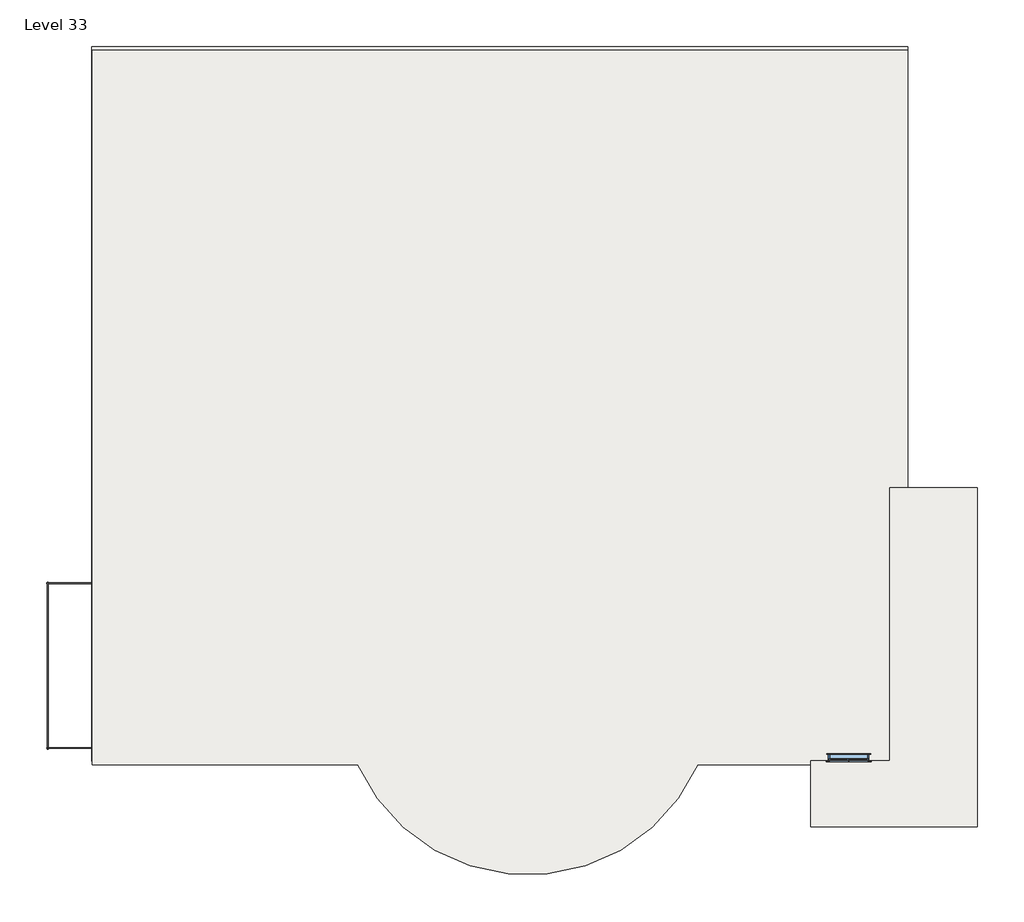
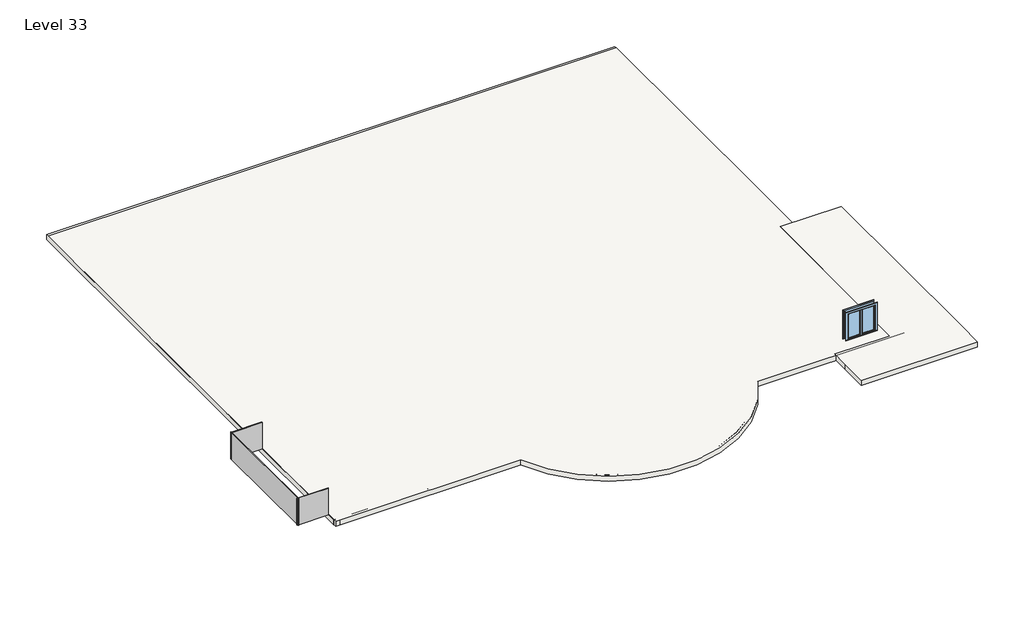
# One storey: 3 plates, 3 slabs, 1 window.
"""IFC4 building model written with IfcOpenShell, lengths in millimetres."""

from ifc_helpers import new_model, si_unit, point, frame, frame_2d, origin, place, context, project, spatial, polyline, circle_curve, trimmed, segment, composite_curve, outline, extrude, transform, mapped, element, save
from components import system_panel_glazed_7d767388, system_panel_glazed_c55d8a5b, window_0862ab64

model = new_model("IFC4")

# Units and contexts
model_context = context("Model", 3, world=origin())
ifc_project = project(units=[si_unit("LENGTHUNIT", "METRE", prefix="MILLI")], contexts=[model_context])

# Site, building, storey
site = spatial("IfcSite", under=ifc_project)
building = spatial("IfcBuilding", under=site)
storey = spatial("IfcBuildingStorey", under=building, Name="Level 33", Elevation=52425.6)

# Plates
placement = place(None, origin())
system_panel_glazed_shape = system_panel_glazed_7d767388(model_context)
element("IfcPlate", 1, ObjectType="System Panel : Glazed", at=placement, inside=storey, context=model_context, shape_type="MappedRepresentation", body=[
    mapped(system_panel_glazed_shape, transform((-17306.4505427, -8690.0239591, 52425.6), x_axis=(-1.0, 0.0, 0.0), y_axis=(0.0, -1.0, 0.0), z_axis=(0.0, 0.0, 1.0))),
])
element("IfcPlate", 2, ObjectType="System Panel : Glazed", at=placement, inside=storey, context=model_context, shape_type="MappedRepresentation", body=[
    mapped(system_panel_glazed_shape, transform((-17306.4505427, -13719.2239591, 52425.6), x_axis=(1.0, 0.0, 0.0), y_axis=(0.0, 1.0, 0.0), z_axis=(0.0, 0.0, 1.0))),
])
system_panel_glazed_2_shape = system_panel_glazed_c55d8a5b(model_context)
element("IfcPlate", 3, ObjectType="System Panel : Glazed", at=placement, inside=storey, context=model_context, shape_type="MappedRepresentation", body=[
    mapped(system_panel_glazed_2_shape, transform((-17979.5505427, -11204.6239591, 52425.6), x_axis=(0.0, -1.0, 0.0), y_axis=(1.0, 0.0, 0.0), z_axis=(0.0, 0.0, 1.0))),
])

# Slabs
element("IfcSlab", 4, ObjectType="9\"", at=placement, inside=storey, context=model_context, shape_type="SweptSolid", body=[
    extrude(outline(composite_curve([segment(polyline([(-16607.9505427, 7350.6120962), (7979.2494573, 7350.6120962), (7979.2494573, -14188.5879038), (1652.8739931, -14188.5879038)]), True, "CONTINUOUS"), segment(trimmed(circle_curve(frame_2d((-3476.1505427, -11898.872104)), 5616.9111737), [point((1652.8739931, -14188.5879038))], [point((-8605.1750786, -14188.5879038))], False, "CARTESIAN"), True, "CONTINUOUS"), segment(polyline([(-8605.1750786, -14188.5879038), (-16404.7505427, -14188.5879038), (-16607.9505427, -14188.5879038), (-16607.9505427, 7350.6120962)]), True, "CONTINUOUS")], self_intersect=False)), frame((0.0, 0.0, 52191.9247039), z_axis=(0.0, 0.0, 1.0), x_axis=(1.0, 0.0, 0.0)), (0.0, 0.0, 1.0), 228.6),
])
element("IfcSlab", 5, ObjectType="9\"", at=placement, inside=storey, context=model_context, shape_type="SweptSolid", body=[
    extrude(outline(composite_curve([segment(polyline([(-16612.6382188, 7457.5128001), (7974.5617812, 7457.5128001), (7974.5617812, -14081.6871999), (1648.1863171, -14081.6871999)]), True, "CONTINUOUS"), segment(trimmed(circle_curve(frame_2d((-3480.8382188, -11791.9714001)), 5616.9111737), [point((1648.1863171, -14081.6871999))], [point((-8609.8627547, -14081.6871999))], False, "CARTESIAN"), True, "CONTINUOUS"), segment(polyline([(-8609.8627547, -14081.6871999), (-16409.4382188, -14081.6871999), (-16612.6382188, -14081.6871999), (-16612.6382188, 7457.5128001)]), True, "CONTINUOUS")], self_intersect=False)), frame((0.0, 0.0, 52190.8232641), z_axis=(0.0, 0.0, 1.0), x_axis=(1.0, 0.0, 0.0)), (0.0, 0.0, 1.0), 228.6),
])
element("IfcSlab", 6, ObjectType="9\"", at=placement, inside=storey, context=model_context, shape_type="SweptSolid", body=[
    extrude(outline(polyline([(5053.3049901, -14840.0808221), (5053.3049901, -14078.0808221), (7237.7049901, -14078.0808221), (7440.9049901, -14078.0808221), (7440.9049901, -5848.4808221), (10082.5049901, -5848.4808221), (10082.5049901, -14840.0808221), (10082.5049901, -16059.2808221), (5053.3049901, -16059.2808221), (5053.3049901, -14840.0808221)])), frame((0.0, 0.0, 52197.0), z_axis=(0.0, 0.0, 1.0), x_axis=(1.0, 0.0, 0.0)), (0.0, 0.0, 1.0), 228.6),
])

# Window
window_shape = window_0862ab64(model_context)
element("IfcWindow", 7, ObjectType="Casement Dbl with Trim : 48\" x 48\"", at=placement, inside=storey, context=model_context, shape_type="MappedRepresentation", body=[
    mapped(window_shape, transform((6201.2494573, -13957.4308221, 51954.0218415), x_axis=(-1.0, 0.0, 0.0), y_axis=(0.0, -1.0, 0.0), z_axis=(0.0, 0.0, 1.0))),
])

save(model, "model.ifc")

# Revit data of these elements
# Type "System Panel : Glazed"
#   Construction Type Id = "GSP4R"
#   Analytic Construction = "1/8 in Pilkington single glazing"
#   Visual Light Transmittance = 0.9
#   Solar Heat Gain Coefficient = 0.86
#   Heat Transfer Coefficient (U) = 1.18115 BTU/(h·ft²·°F)
# Type "9\""
#   Assembly Code = "B1010"
#   Function = 0
#   Layers, outside or top first: 0' - 9" no material (function 1)
# Type "Casement Dbl with Trim : 48\" x 48\""
#   Type Mark = "10"
#   Construction Type Id = "GSP4R"
#   Assembly Code = "B2020100"
#   Analytic Construction = "1/8 in Pilkington single glazing"
#   Visual Light Transmittance = 0.9
#   Solar Heat Gain Coefficient = 0.78
#   Heat Transfer Coefficient (U) = 0.6496 BTU/(h·ft²·°F)
#   Height = 4' - 0"
#   Default Sill Height = 3' - 0"
#   Trim Projection - Ext. = 0' - 0 1/2"
#   Trim Projection - Int. = 0' - 0 3/4"
#   Trim Width - Exterior = 0' - 3 1/2"
#   Trim Width - Interior = 0' - 3 1/2"
#   Width = 4' - 0"
#   Window Inset = 0' - 0 3/4"
#   Define Thermal Properties by = 1
#   Glass Pane Material = Glass
#   Sash Material = Sash
#   Trim Exterior Material = Trim
#   Trim Interior Material = Trim
#   Wall Closure = (empty or 0)
# Elements 1, 2, 3 (IfcPlate, "System Panel : Glazed")
#   Phase Created = New Construction
#   Materials on its faces: "Glass"
# Element 4 (IfcSlab, "9\"")
#   built-in parameter 1001955 = 1.5708 (stored number, unit not read)
#   Height Offset From Level = -0' - 0.19981"
#   Phase Created = New Construction
#   Materials on its faces: "Default Floor"
# Element 5 (IfcSlab, "9\"")
#   built-in parameter 1001955 = 1.5708 (stored number, unit not read)
#   Height Offset From Level = -0' - 0.24318"
#   Phase Created = New Construction
#   Materials on its faces: "Default Floor"
# Element 6 (IfcSlab, "9\"")
#   built-in parameter 1001955 = -1.5708 (stored number, unit not read)
#   Height Offset From Level = 0' - 0"
#   Phase Created = New Construction
#   Materials on its faces: "Default Floor"
# Element 7 (IfcWindow, "Casement Dbl with Trim : 48\" x 48\"")
#   Mark = "45"
#   Phase Created = New Construction
#   Materials on its faces: "Sash", "Trim", "Glass"
# Materials
#   "Glass": class "Glass", colour RGB 0 128 192, transparency 0.75, Description = "Soda Lime Glass", Cost = 0
#   "Sash": class "Wood", colour RGB 224 178 126, transparency 0
#   "Trim": class "Wood", colour RGB 224 178 126, transparency 0
#   "Default Floor": colour RGB 128 128 128, transparency 0
